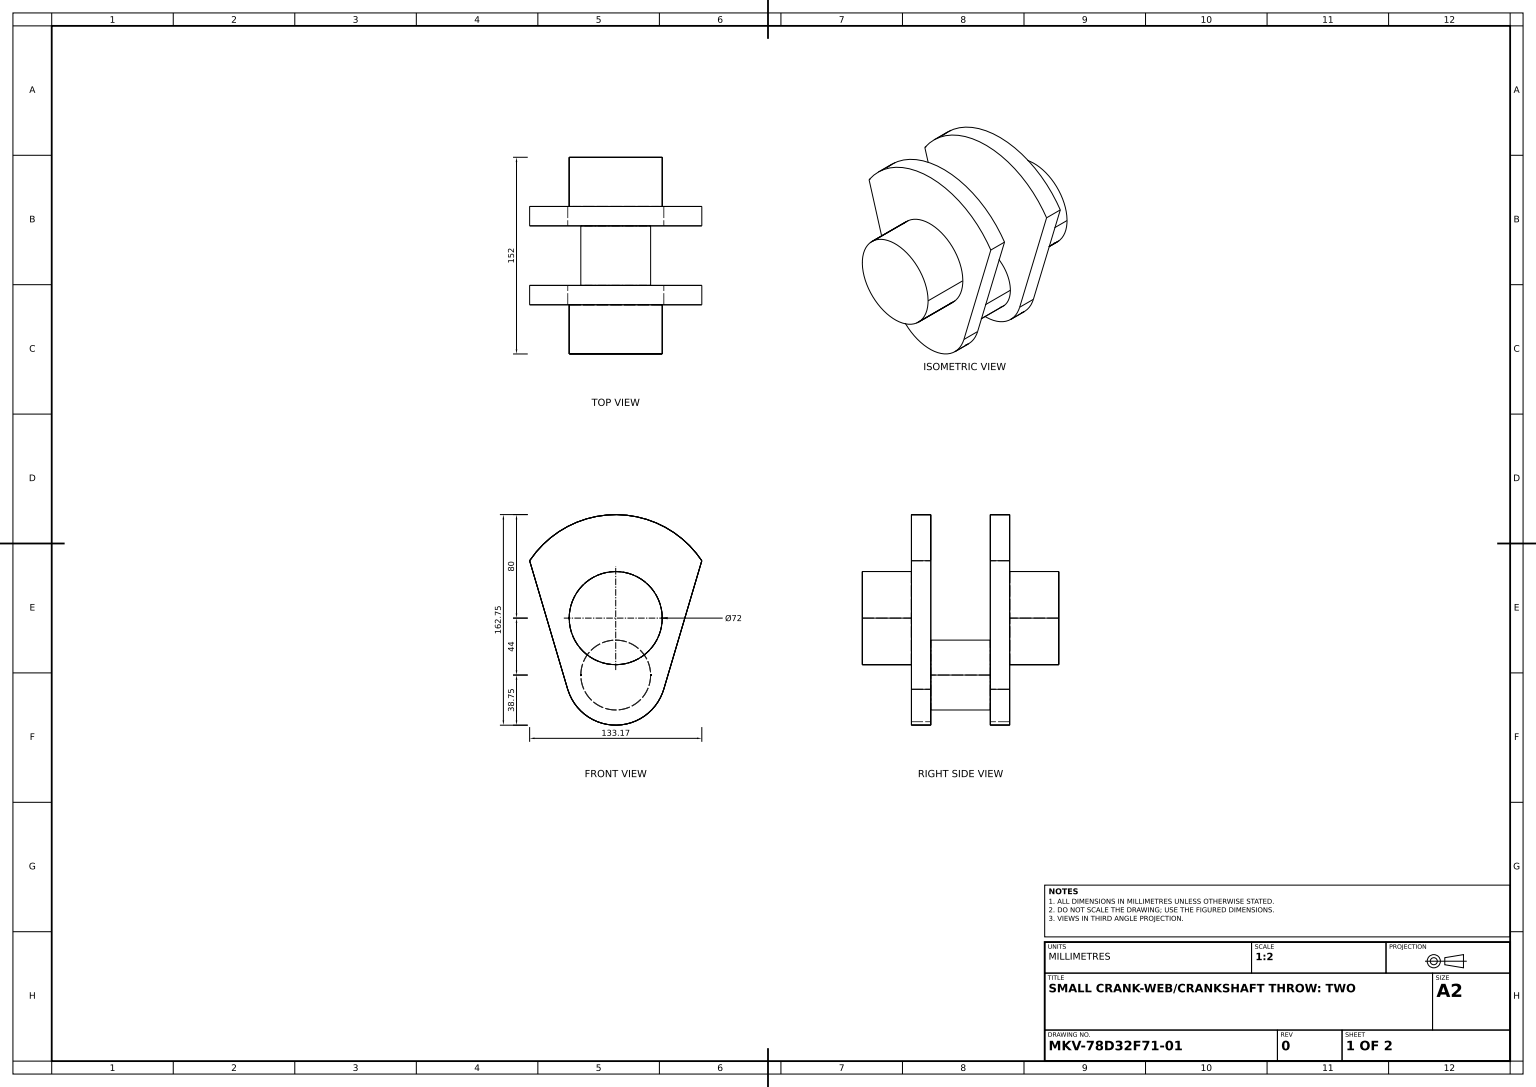
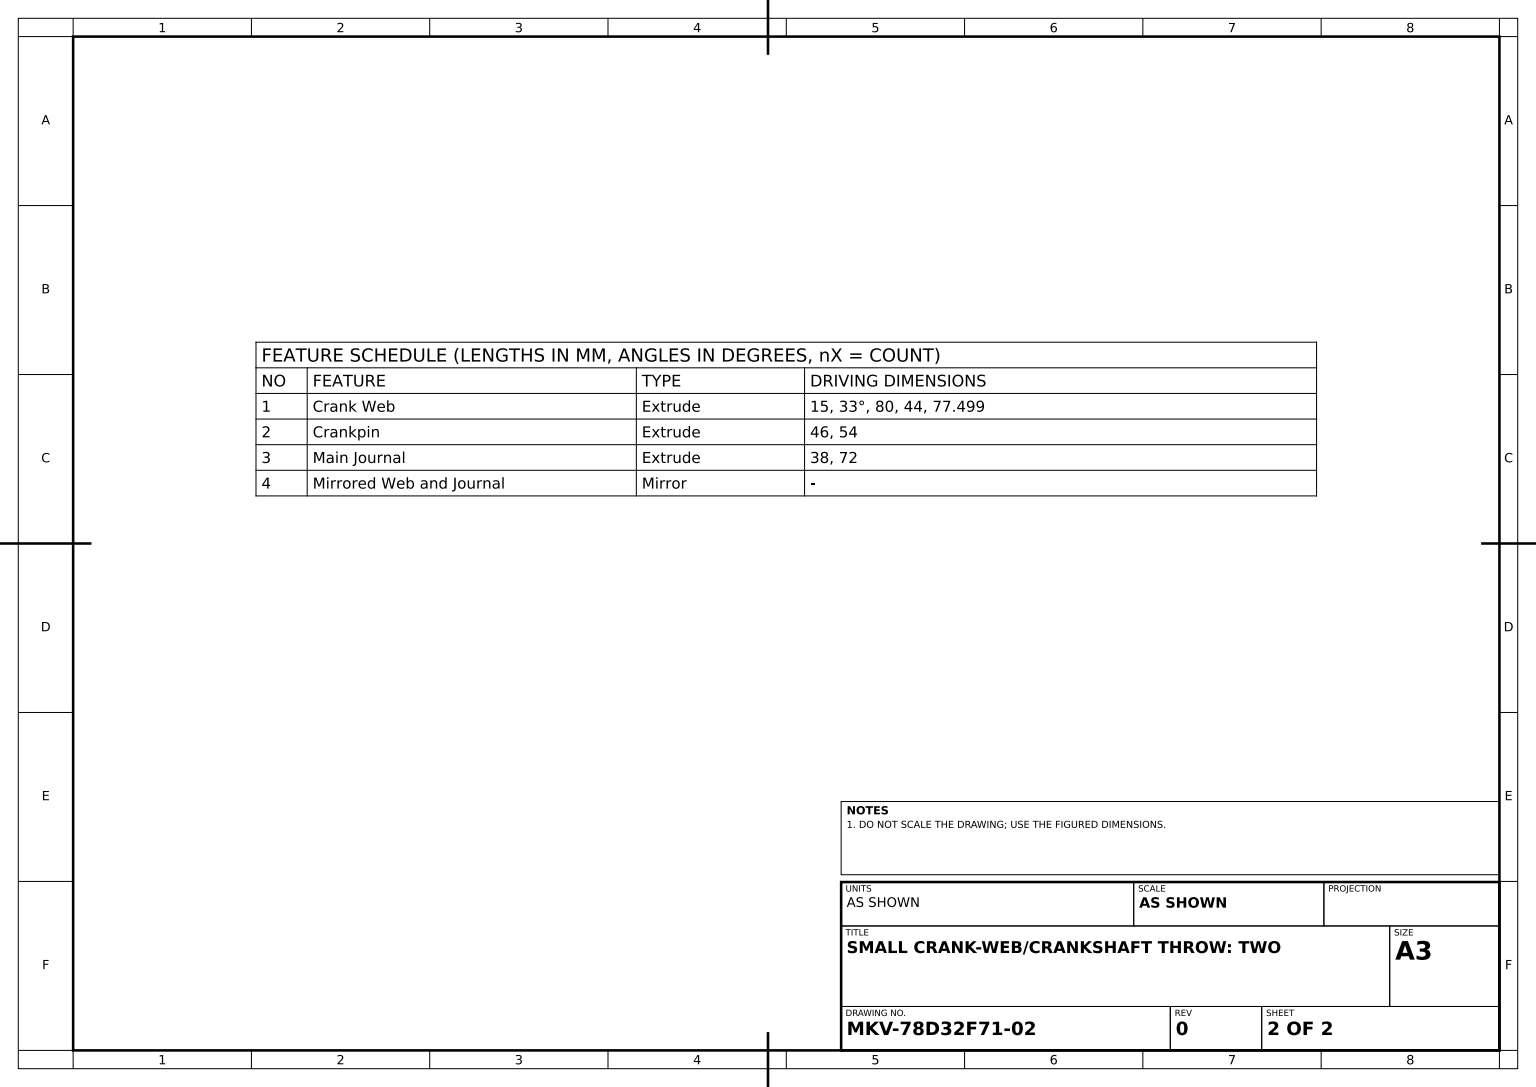
SolidWorks part; units mm, degrees
material "Plain Carbon Steel"
ref_plane "Front Plane" through (0, 0, 0) normal (0, 0, 1) x (1, 0, 0)
ref_plane "Top Plane" through (0, 0, 0) normal (0, 1, 0) x (1, 0, 0)
ref_plane "Right Plane" through (0, 0, 0) normal (1, 0, 0) x (0, 0, -1)
sketch "Crank Web Profile" plane through (0, 0, 0) normal (0, 0, 1) x (1, 0, 0)
  line L0 (0, 80.8512) -> (0, -44) construction
  line L1 (-50.3754, 0) -> (95.4628, 0) construction
  line L2 (-66.5833, 44.3471) -> (-37.1538, -55.0054)
  line L3 (66.5833, 44.3471) -> (37.1538, -55.0054)
  circle A0 centre (0, -44) radius 38.7495
  arc A1 (-66.5833, 44.3471) -> (66.5833, 44.3471) centre (0, 0) cw
  dimension "D1" = 33
  dimension "D2" = 80
  dimension "D4" = 77.499
  dimension "D3" = 44
extrude "Crank Web" add sketch "Crank Web Profile" along normal blind 15 contours A1 L2 A0 L3 | A0 L0
sketch "Crankpin Profile" plane through (0, 0, 0) normal (0, 0, -1) x (-1, 0, 0)
  circle A0 centre (0, -44) radius 27
  dimension "D1" = 54
extrude "Crankpin" add sketch "Crankpin Profile" along normal blind 46
sketch "Main Journal Profile" plane through (0, 0, 15) normal (0, 0, 1) x (1, 0, 0)
  circle A0 centre (0, 0) radius 36
  dimension "D1" = 72
extrude "Main Journal" add sketch "Main Journal Profile" along normal blind 38
ref_plane "Crankpin Mid Plane" through (0, 0, -23) normal (0, 0, -1) x (-1, 0, 0)
mirror "Mirrored Web and Journal" about plane through (0, 0, -23) normal (0, 0, -1) of "Crank Web", "Main Journal"
ref_plane "Crank Reference Plane" through (0, 0, -80) normal (0, 0, -1) x (-1, 0, 0)
